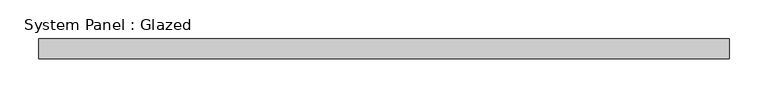
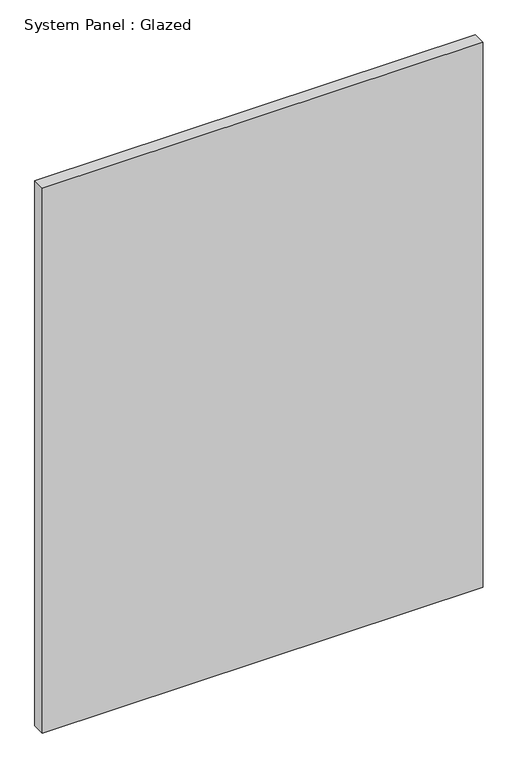
"""IFC4 building model written with IfcOpenShell, lengths in millimetres: plate geometry, System Panel : Glazed."""

from ifc_helpers import new_model, si_unit, origin, origin_with_axes, place, context, project, spatial, polyline, outline, extrude, source, transform, mapped, element, save


def system_panel_glazed_3b0fd0dd(model_context):
    return source(origin(), model_context, "Body", "SweptSolid", [
        extrude(outline(polyline([(442.3582878, 19.05), (-442.3582878, 19.05), (-442.3582878, 44.45), (442.3582878, 44.45), (442.3582878, 19.05)])), origin_with_axes(), (0.0, 0.0, 1.0), 1155.7),
    ])


if __name__ == "__main__":
    model = new_model("IFC4")
    model_context = context("Model", 3, world=origin())
    ifc_project = project(units=[si_unit("LENGTHUNIT", "METRE", prefix="MILLI")], contexts=[model_context])
    site = spatial("IfcSite", under=ifc_project)
    building = spatial("IfcBuilding", under=site)
    placement = place(None, origin())
    system_panel_glazed_shape = system_panel_glazed_3b0fd0dd(model_context)
    element("IfcPlate", 1, ObjectType="System Panel : Glazed", at=placement, inside=building, context=model_context, shape_type="MappedRepresentation", body=[
        mapped(system_panel_glazed_shape, transform((0.0, 0.0, 0.0), x_axis=(1.0, 0.0, 0.0), y_axis=(0.0, 1.0, 0.0), z_axis=(0.0, 0.0, 1.0))),
    ])
    save(model, "model.ifc")

# Revit data of these elements
# Type "System Panel : Glazed"
#   Construction Type Id = "GSP4R"
#   Analytic Construction = "1/8 in Pilkington single glazing"
#   Visual Light Transmittance = 0.9
#   Solar Heat Gain Coefficient = 0.86
#   Heat Transfer Coefficient (U) = 1.18115 BTU/(h·ft²·°F)
# Element 1 (IfcPlate, "System Panel : Glazed")
#   Materials on its faces: "Glass"
# Materials
#   "Glass": class "Glass", colour RGB 0 128 192, transparency 0.75, Description = "Soda Lime Glass", Cost = 0
